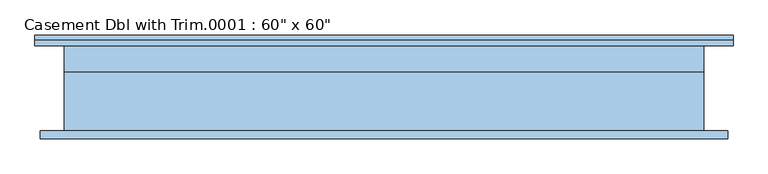
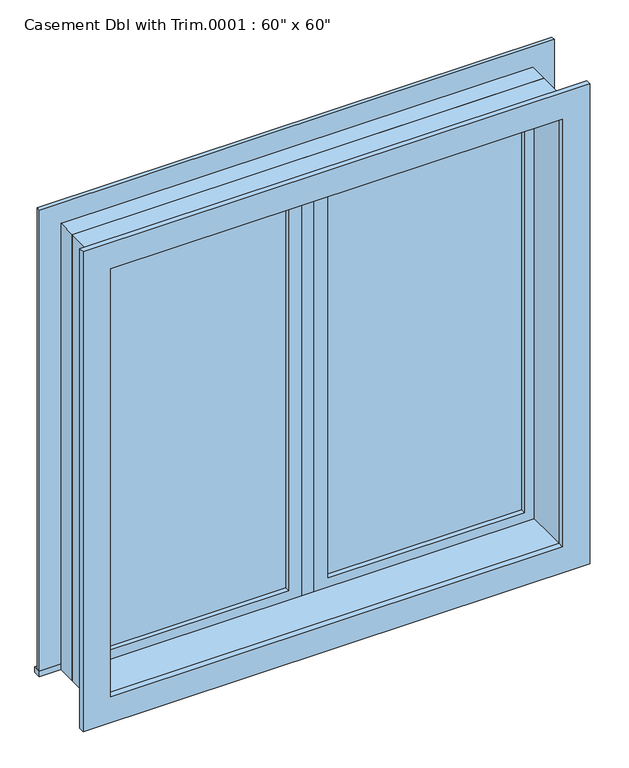
"""IFC4 building model written with IfcOpenShell, lengths in millimetres: window geometry."""

from ifc_helpers import new_model, si_unit, frame, origin, place, context, project, spatial, polyline, outline, extrude, source, transform, mapped, element, save


def window_514a67b1(model_context):
    return source(origin(), model_context, "Body", "SweptSolid", [
        extrude(outline(polyline([(63.5, 85.725), (698.5, 85.725), (698.5, 73.025), (63.5, 73.025), (63.5, 85.725)])), frame((0.0, 0.0, 977.9), z_axis=(0.0, 0.0, 1.0), x_axis=(1.0, 0.0, 0.0)), (0.0, 0.0, 1.0), 1397.0),
        extrude(outline(polyline([(2419.35, 19.05), (933.45, 19.05), (933.45, 742.95), (2419.35, 742.95), (2419.35, 19.05)]), holes=[polyline([(2374.9, 63.5), (2374.9, 698.5), (977.9, 698.5), (977.9, 63.5), (2374.9, 63.5)])]), frame((0.0, 57.15, 0.0), z_axis=(0.0, 1.0, 0.0), x_axis=(0.0, 0.0, 1.0)), (0.0, 0.0, 1.0), 44.45),
        extrude(outline(polyline([(19.05, 57.15), (-19.05, 57.15), (-19.05, 120.65), (19.05, 120.65), (19.05, 57.15)])), frame((0.0, 0.0, 933.45), z_axis=(0.0, 0.0, 1.0), x_axis=(1.0, 0.0, 0.0)), (0.0, 0.0, 1.0), 1485.9),
        extrude(outline(polyline([(-831.85, 146.05), (831.85, 146.05), (831.85, 120.65), (-831.85, 120.65), (-831.85, 146.05)])), frame((0.0, 0.0, 914.4), z_axis=(0.0, 0.0, 1.0), x_axis=(1.0, 0.0, 0.0)), (0.0, 0.0, 1.0), 19.05),
        extrude(outline(polyline([(2419.35, -742.95), (2419.35, 742.95), (933.45, 742.95), (933.45, 831.85), (2508.25, 831.85), (2508.25, -831.85), (933.45, -831.85), (933.45, -742.95), (2419.35, -742.95)])), frame((0.0, 120.65, 0.0), z_axis=(0.0, 1.0, 0.0), x_axis=(0.0, 0.0, 1.0)), (0.0, 0.0, 1.0), 12.7),
        extrude(outline(polyline([(2495.55, 819.15), (2495.55, -819.15), (857.25, -819.15), (857.25, 819.15), (2495.55, 819.15)]), holes=[polyline([(2406.65, 730.25), (946.15, 730.25), (946.15, -730.25), (2406.65, -730.25), (2406.65, 730.25)])]), frame((0.0, -101.6, 0.0), z_axis=(0.0, 1.0, 0.0), x_axis=(0.0, 0.0, 1.0)), (0.0, 0.0, 1.0), 19.05),
        extrude(outline(polyline([(-63.5, 73.025), (-698.5, 73.025), (-698.5, 85.725), (-63.5, 85.725), (-63.5, 73.025)])), frame((0.0, 0.0, 977.9), z_axis=(0.0, 0.0, 1.0), x_axis=(1.0, 0.0, 0.0)), (0.0, 0.0, 1.0), 1397.0),
        extrude(outline(polyline([(2419.35, -742.95), (933.45, -742.95), (933.45, -19.05), (2419.35, -19.05), (2419.35, -742.95)]), holes=[polyline([(2374.9, -698.5), (2374.9, -63.5), (977.9, -63.5), (977.9, -698.5), (2374.9, -698.5)])]), frame((0.0, 57.15, 0.0), z_axis=(0.0, 1.0, 0.0), x_axis=(0.0, 0.0, 1.0)), (0.0, 0.0, 1.0), 44.45),
        extrude(outline(polyline([(2438.4, -762.0), (914.4, -762.0), (914.4, 762.0), (2438.4, 762.0), (2438.4, -762.0)]), holes=[polyline([(2406.65, -730.25), (2406.65, 730.25), (946.15, 730.25), (946.15, -730.25), (2406.65, -730.25)])]), frame((0.0, -82.55, 0.0), z_axis=(0.0, 1.0, 0.0), x_axis=(0.0, 0.0, 1.0)), (0.0, 0.0, 1.0), 139.7),
        extrude(outline(polyline([(2438.4, 762.0), (2438.4, -762.0), (914.4, -762.0), (914.4, 762.0), (2438.4, 762.0)]), holes=[polyline([(2419.35, 742.95), (933.45, 742.95), (933.45, -742.95), (2419.35, -742.95), (2419.35, 742.95)])]), frame((0.0, 57.15, 0.0), z_axis=(0.0, 1.0, 0.0), x_axis=(0.0, 0.0, 1.0)), (0.0, 0.0, 1.0), 63.5),
    ])


if __name__ == "__main__":
    model = new_model("IFC4")
    model_context = context("Model", 3, world=origin())
    ifc_project = project(units=[si_unit("LENGTHUNIT", "METRE", prefix="MILLI")], contexts=[model_context])
    site = spatial("IfcSite", under=ifc_project)
    building = spatial("IfcBuilding", under=site)
    placement = place(None, origin())
    window_shape = window_514a67b1(model_context)
    element("IfcWindow", 1, ObjectType="Casement Dbl with Trim.0001 : 60\" x 60\"", at=placement, inside=building, context=model_context, shape_type="MappedRepresentation", body=[
        mapped(window_shape, transform((0.0, 0.0, 0.0), x_axis=(1.0, 0.0, 0.0), y_axis=(0.0, 1.0, 0.0), z_axis=(0.0, 0.0, 1.0))),
    ])
    save(model, "model.ifc")

# Revit data of these elements
# Type "Casement Dbl with Trim.0001 : 60\" x 60\""
#   Type Mark = "10"
#   Construction Type Id = "GSP4R"
#   Assembly Code = "B2020100"
#   Analytic Construction = "1/8 in Pilkington single glazing"
#   Visual Light Transmittance = 0.9
#   Solar Heat Gain Coefficient = 0.78
#   Heat Transfer Coefficient (U) = 0.6496 BTU/(h·ft²·°F)
#   Height = 5' - 0"
#   Default Sill Height = 3' - 0"
#   Trim Projection - Ext. = 0' - 0 1/2"
#   Trim Projection - Int. = 0' - 0 3/4"
#   Trim Width - Exterior = 0' - 3 1/2"
#   Trim Width - Interior = 0' - 3 1/2"
#   Width = 5' - 0"
#   Window Inset = 0' - 0 3/4"
#   Define Thermal Properties by = 1
#   Glass Pane Material = Glass
#   Sash Material = Sash
#   Trim Exterior Material = Trim
#   Trim Interior Material = Trim
#   Wall Closure = (empty or 0)
# Element 1 (IfcWindow, "Casement Dbl with Trim.0001 : 60\" x 60\"")
#   Materials on its faces: "Sash", "Trim", "Glass"
# Materials
#   "Glass": class "Glass", colour RGB 0 128 192, transparency 0.75, Description = "Soda Lime Glass", Cost = 0
#   "Sash": class "Wood", colour RGB 224 178 126, transparency 0
#   "Trim": class "Wood", colour RGB 224 178 126, transparency 0
